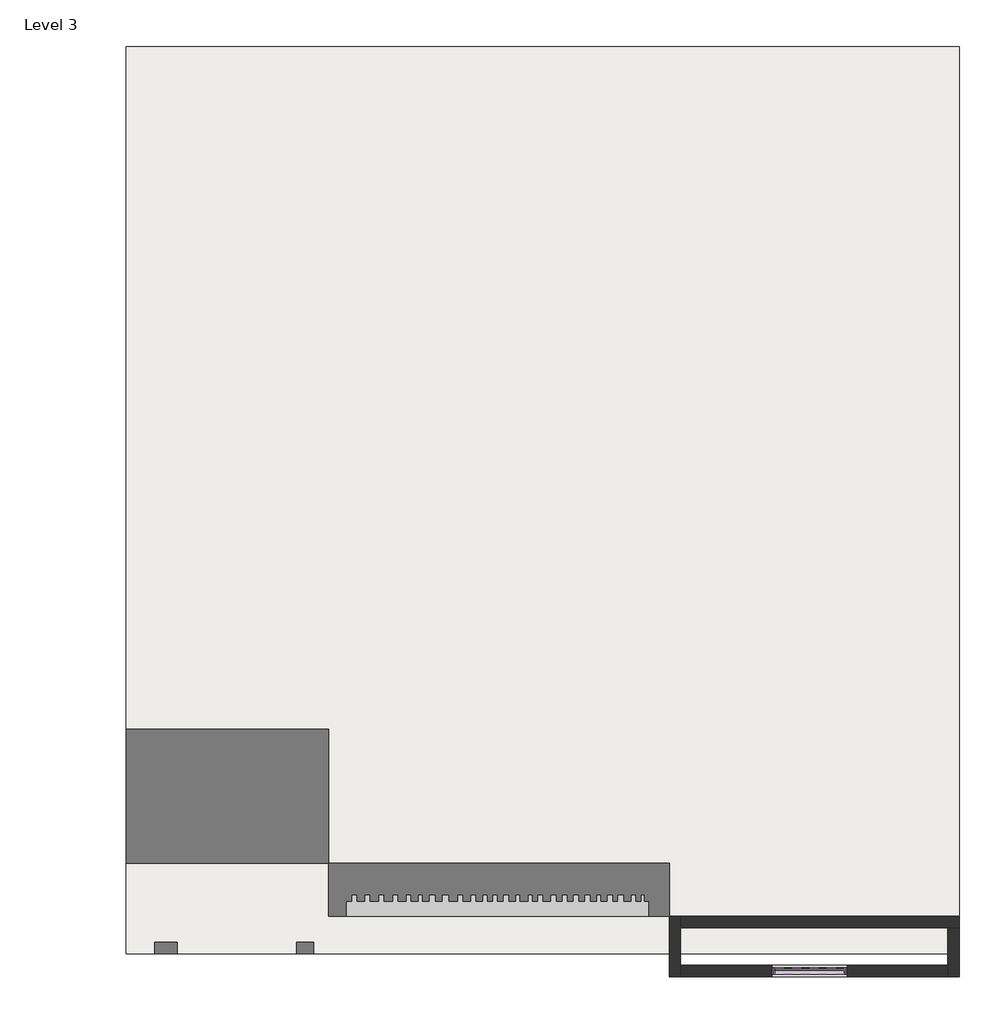
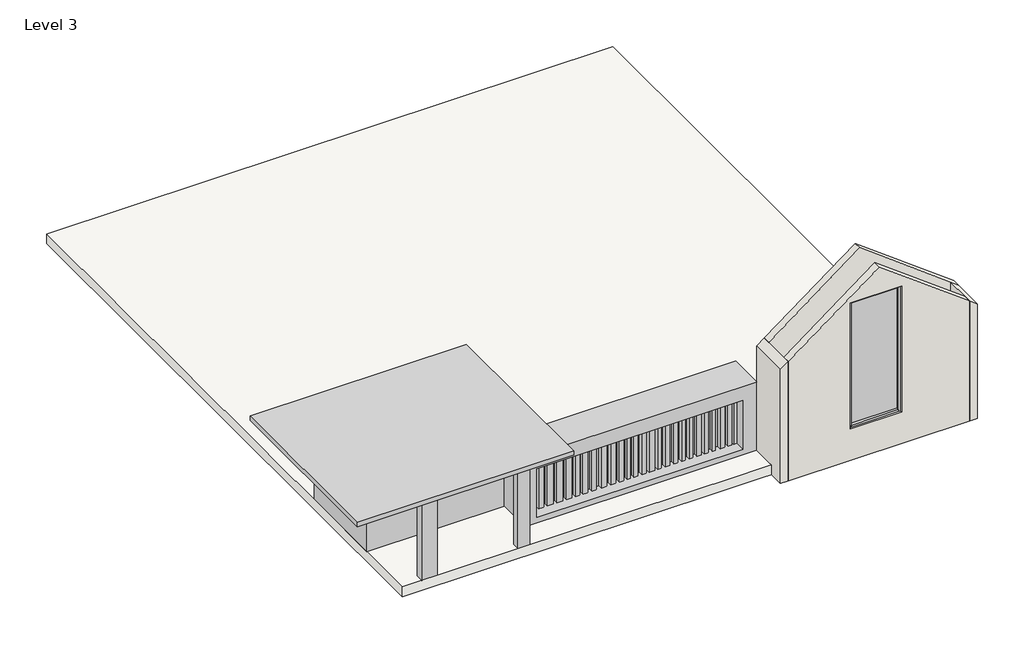
# One storey: 4 members, 4 walls, 1 plate, 1 proxy, 1 roof.
"""IFC4 building model written with IfcOpenShell, lengths in millimetres."""

from ifc_helpers import new_model, si_unit, frame, origin, place, context, project, spatial, polyline, outline, extrude, faceted_brep, transform, mapped, element, save
from components import generic_models_4_generic_models_4_f36dcc8b, member_f07b7441, member_fc36c840, system_panel_glazed_b761a9a7

model = new_model("IFC4")

# Units and contexts
model_context = context("Model", 3, world=origin())
ifc_project = project(units=[si_unit("LENGTHUNIT", "METRE", prefix="MILLI")], contexts=[model_context])

# Site, building, storey
site = spatial("IfcSite", under=ifc_project)
building = spatial("IfcBuilding", under=site)
storey = spatial("IfcBuildingStorey", under=building, Name="Level 3", Elevation=6096.0)

# Proxy
placement = place(None, origin())
generic_models_4_generic_models_4_shape = generic_models_4_generic_models_4_f36dcc8b(model_context)
element("IfcBuildingElementProxy", 1, Name="Generic Models 4 : Generic Models 4", ObjectType="Generic Models 4 : Generic Models 4", at=placement, inside=storey, context=model_context, shape_type="MappedRepresentation", body=[
    mapped(generic_models_4_generic_models_4_shape, transform((0.0, 0.0, 0.0), x_axis=(1.0, 0.0, 0.0), y_axis=(0.0, 1.0, 0.0), z_axis=(0.0, 0.0, 1.0))),
])

# Members
member_shape = member_f07b7441(model_context)
element("IfcMember", 2, ObjectType="Rectangular Mullion : 2.5\" x 5\" rectangular", at=placement, inside=storey, context=model_context, shape_type="MappedRepresentation", body=[
    mapped(member_shape, transform((11442.039189, -13725.5436591, 11036.2085927), x_axis=(0.0, 0.0, 1.0), y_axis=(0.0, -1.0, 0.0), z_axis=(1.0, 0.0, 0.0))),
])
element("IfcMember", 3, ObjectType="Rectangular Mullion : 2.5\" x 5\" rectangular", at=placement, inside=storey, context=model_context, shape_type="MappedRepresentation", body=[
    mapped(member_shape, transform((10045.039189, -13725.5436591, 7084.9880738), x_axis=(0.0, 0.0, -1.0), y_axis=(0.0, -1.0, 0.0), z_axis=(-1.0, 0.0, 0.0))),
])
member_2_shape = member_fc36c840(model_context)
element("IfcMember", 4, ObjectType="Rectangular Mullion : 2.5\" x 5\" rectangular", at=placement, inside=storey, context=model_context, shape_type="MappedRepresentation", body=[
    mapped(member_2_shape, transform((9981.539189, -13725.5436591, 11036.2085927), x_axis=(-1.0, 0.0, 0.0), y_axis=(0.0, -1.0, 0.0), z_axis=(0.0, 0.0, 1.0))),
])
element("IfcMember", 5, ObjectType="Rectangular Mullion : 2.5\" x 5\" rectangular", at=placement, inside=storey, context=model_context, shape_type="MappedRepresentation", body=[
    mapped(member_2_shape, transform((11505.539189, -13725.5436591, 7084.9880738), x_axis=(1.0, 0.0, 0.0), y_axis=(0.0, -1.0, 0.0), z_axis=(0.0, 0.0, -1.0))),
])

# Plate
system_panel_glazed_shape = system_panel_glazed_b761a9a7(model_context)
element("IfcPlate", 6, ObjectType="System Panel : Glazed", at=placement, inside=storey, context=model_context, shape_type="MappedRepresentation", body=[
    mapped(system_panel_glazed_shape, transform((10743.539189, -13725.5436591, 7148.4880738), x_axis=(1.0, 0.0, 0.0), y_axis=(0.0, 1.0, 0.0), z_axis=(0.0, 0.0, 1.0))),
])

# Roof
element("IfcRoof", 7, ObjectType="Generic - 12\"", at=placement, inside=storey, context=model_context, shape_type="SweptSolid", body=[
    extrude(outline(polyline([(-3010.560811, 4873.4397401), (13753.439189, 4873.4397401), (13753.439189, -13376.4602599), (-3010.560811, -13376.4602599), (-3010.560811, 4873.4397401)])), frame((0.0, 0.0, 6096.0), z_axis=(0.0, 0.0, 1.0), x_axis=(1.0, 0.0, 0.0)), (0.0, 0.0, 1.0), 304.8),
])

# Walls
element("IfcWall", 8, ObjectType="9\"", at=placement, inside=storey, context=model_context, shape_type="Brep", body=[
    faceted_brep([(8144.7030034, -13839.8436591, 6096.0), (8144.7030034, -13611.2436591, 6096.0), (8144.7030034, -12849.2436591, 6096.0), (8144.7030034, -12620.6436591, 6096.0), (8144.7030034, -12620.6436591, 9837.134627), (8144.7030034, -12849.2436591, 9837.134627), (8144.7030034, -13611.2436591, 9837.134627), (8144.7030034, -13839.8436591, 9837.134627), (7916.1030034, -13839.8436591, 6096.0), (7916.1030034, -13839.8436591, 9665.684627), (7916.1030034, -12620.6436591, 9665.684627), (7916.1030034, -12620.6436591, 6096.0)], [[[0, 1, 2, 3, 4, 5, 6, 7]], [[8, 9, 10, 11]], [[3, 2, 1, 0, 8, 11]], [[4, 3, 11, 10]], [[0, 7, 9, 8]], [[7, 6, 5, 4, 10, 9]]]),
])
element("IfcWall", 9, ObjectType="9\"", at=placement, inside=storey, context=model_context, shape_type="Brep", body=[
    faceted_brep([(8144.7030034, -12849.2436591, 6096.0), (13524.839189, -12849.2436591, 6096.0), (13753.439189, -12849.2436591, 6096.0), (13753.439189, -12849.2436591, 9678.6297298), (13524.839189, -12849.2436591, 9850.0797298), (10843.4011647, -12849.2436591, 11861.158248), (8144.7030034, -12849.2436591, 9837.134627), (8144.7030034, -12620.6436591, 6096.0), (8144.7030034, -12620.6436591, 9837.134627), (10843.4011647, -12620.6436591, 11861.158248), (13753.439189, -12620.6436591, 9678.6297298), (13753.439189, -12620.6436591, 6096.0)], [[[0, 1, 2, 3, 4, 5, 6]], [[7, 8, 9, 10, 11]], [[0, 6, 8, 7]], [[3, 2, 11, 10]], [[2, 1, 0, 7, 11]], [[6, 5, 9, 8]], [[5, 4, 3, 10, 9]]]),
])
element("IfcWall", 10, ObjectType="9\"", at=placement, inside=storey, context=model_context, shape_type="Brep", body=[
    faceted_brep([(13524.839189, -12849.2436591, 6096.0), (13524.839189, -13611.2436591, 6096.0), (13524.839189, -13839.8436591, 6096.0), (13524.839189, -13839.8436591, 9850.0797298), (13524.839189, -13611.2436591, 9850.0797298), (13524.839189, -12849.2436591, 9850.0797298), (13753.439189, -12849.2436591, 6096.0), (13753.439189, -12849.2436591, 9678.6297298), (13753.439189, -13839.8436591, 9678.6297298), (13753.439189, -13839.8436591, 6096.0)], [[[0, 1, 2, 3, 4, 5]], [[6, 7, 8, 9]], [[2, 1, 0, 6, 9]], [[0, 5, 7, 6]], [[3, 2, 9, 8]], [[5, 4, 3, 8, 7]]]),
])
element("IfcWall", 11, ObjectType="9\"", at=placement, inside=storey, context=model_context, shape_type="SweptSolid", body=[
    extrude(outline(polyline([(6096.0, 8144.7030034), (6096.0, 13524.839189), (9850.0797298, 13524.839189), (11861.158248, 10843.4011647), (9837.134627, 8144.7030034), (6096.0, 8144.7030034)]), holes=[polyline([(7084.9880738, 9981.539189), (11036.2085927, 9981.539189), (11036.2085927, 11505.539189), (7084.9880738, 11505.539189), (7084.9880738, 9981.539189)])]), frame((0.0, -13839.8436591, 0.0), z_axis=(0.0, 1.0, 0.0), x_axis=(0.0, 0.0, 1.0)), (0.0, 0.0, 1.0), 228.6),
])

save(model, "model.ifc")

# Revit data of these elements
# Type "Rectangular Mullion : 2.5\" x 5\" rectangular"
#   built-in parameter 1007304 = 0.416667 (stored number, unit not read)
#   built-in parameter 1007301 = 0.104167 (stored number, unit not read)
#   built-in parameter 1007300 = 0.104167 (stored number, unit not read)
# Type "System Panel : Glazed"
#   Construction Type Id = "GSP4R"
#   Analytic Construction = "1/8 in Pilkington single glazing"
#   Visual Light Transmittance = 0.9
#   Solar Heat Gain Coefficient = 0.86
#   Heat Transfer Coefficient (U) = 1.18115 BTU/(h·ft²·°F)
#   Define Thermal Properties by = 1
# Type "Generic - 12\""
#   Assembly Code = "B1020"
#   Layers, outside or top first: 1' - 0" no material (function 1)
# Type "9\""
#   Assembly Code = "B2010"
#   Layers, outside or top first: 0' - 9" no material (function 1)
# Element 1 (IfcBuildingElementProxy, "Generic Models 4 : Generic Models 4")
#   Phase Created = New Construction
# Elements 2, 3, 4, 5 (IfcMember, "Rectangular Mullion : 2.5\" x 5\" rectangular")
#   Phase Created = New Construction
#   Materials on its faces: "Aluminum"
# Element 6 (IfcPlate, "System Panel : Glazed")
#   Phase Created = New Construction
#   Materials on its faces: "Glass"
# Element 7 (IfcRoof, "Generic - 12\"")
#   built-in parameter 1001705 = 21 (stored number, unit not read)
#   built-in parameter 1001710 = 33615
#   Phase Created = New Construction
#   Materials on its faces: "Default Roof"
# Elements 8, 9, 10, 11 (IfcWall, "9\"")
#   Top Offset = 0' - 0"
#   Base Offset = 0' - 0"
#   Unconnected Height = 10' - 0"
#   wall height = 10' - 0"
#   Phase Created = New Construction
#   Base Constraint = Level 3
#   Materials on its faces: "Default Wall"
# Materials
#   "Aluminum": class "Metal", colour RGB 247 247 247, transparency 0, Description = "Aluminum 6061", Cost = 0
#   "Glass": class "Glass", colour RGB 0 128 192, transparency 0.75, Description = "Soda Lime Glass", Cost = 0
#   "Default Roof": colour RGB 88 101 114, transparency 0, Cost = 0
#   "Default Wall": colour RGB 128 128 128, transparency 0, Cost = 0
